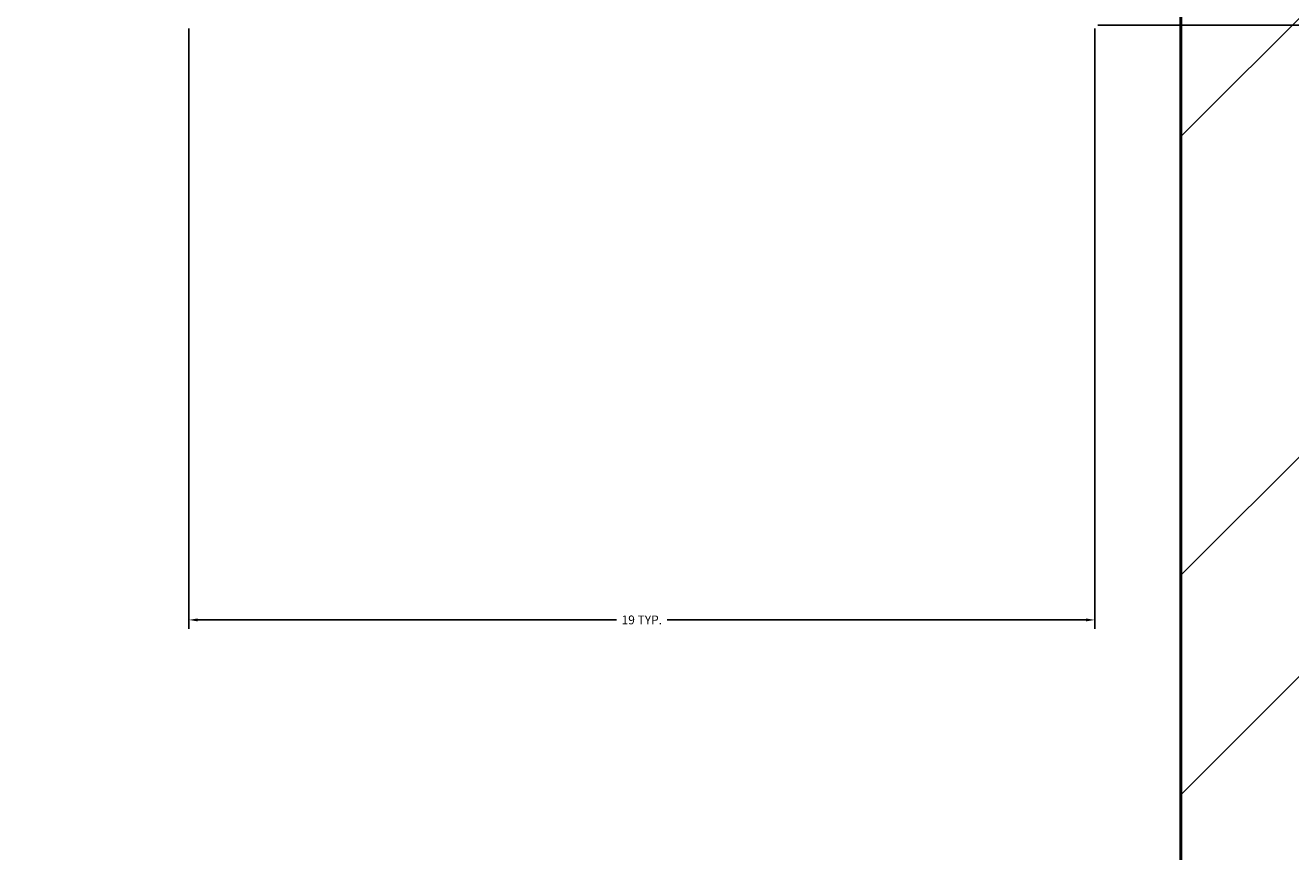
# Model space of a CAD drawing. Units: inches. Extents: x 963 to 2075, y 289 to 2657.
# Tile 20 of 98: x 1485 to 1511, y 1718 to 1735. Entities that reach past the tile are written whole.
import ezdxf

# ---------------------------------------------------------------- set-up
doc = ezdxf.new("R2010")
doc.units = ezdxf.units.IN
for name, color, linetype, lineweight in [('A-ANNO-DIMS', 2, 'Continuous', 18), ('A-WALL', 7, 'Continuous', 50), ('A-WALL-PATT', 8, 'Continuous', 13)]:
    doc.layers.add(name, color=color, linetype=linetype, lineweight=lineweight)
doc.styles.get("Standard").update_dxf_attribs({"font": 'arial.ttf'})
doc.dimstyles.get("Standard").update_dxf_attribs({"dimtxt": 0.18, "dimasz": 0.18, "dimexe": 0.18, "dimexo": 0.0625, "dimgap": 0.09, "dimtad": 0, "dimtih": 1, "dimtoh": 1, "dimdec": 4, "dimzin": 0, "dimdsep": 46, "dimtxsty": 'Standard', "dimcen": 0.09, "dimadec": 0, "dimazin": 0, "dimtfac": 1, "dimtdec": 4, "dimtofl": 0, "dimtmove": 0, "dimatfit": 3, "dimfxl": 1, "dimtolj": 1, "dimtzin": 0, "dimarcsym": 0})

# ---------------------------------------------------------------- blocks, each defined once
blk = doc.blocks.new('*D28')
at = {"layer": 'A-ANNO-DIMS', "color": 0, "lineweight": -2, "transparency": 16777216}
for p, q in [((1506.727, 1816.319), (1519.012, 1816.319)), ((1518.832, 1816.139), (1518.832, 1775.944)), ((1518.832, 1735.382), (1518.832, 1775.577)), ((1506.727, 1735.202), (1519.012, 1735.202))]:
    blk.add_line(p, q, dxfattribs=at)
at = {"layer": 'A-ANNO-DIMS', "color": 0, "transparency": 16777216}
for points in [[(1518.802, 1816.139), (1518.862, 1816.139), (1518.832, 1816.319)], [(1518.802, 1735.382), (1518.862, 1735.382), (1518.832, 1735.202)]]:
    blk.add_solid(points, dxfattribs=at)
at = {"layer": 'Defpoints', "color": 0, "transparency": 16777216}
for p in [(1506.665, 1816.319), (1518.832, 1816.319), (1506.665, 1735.202)]:
    blk.add_point(p, dxfattribs=at)
at = {"layer": 'A-ANNO-DIMS', "color": 0, "transparency": 16777216, "insert": (1518.832, 1775.761), "char_height": 0.18, "attachment_point": 5}
blk.add_mtext('\\A1;3-SEAT SOFA 81 TYP.', dxfattribs=at)
blk = doc.blocks.new('*D29')
at = {"layer": 'A-ANNO-DIMS', "color": 0, "lineweight": -2, "transparency": 16777216}
for p, q in [((1488.124, 1735.14), (1488.124, 1722.855)), ((1506.665, 1735.14), (1506.665, 1722.855)), ((1488.304, 1723.035), (1496.875, 1723.035)), ((1506.485, 1723.035), (1497.914, 1723.035))]:
    blk.add_line(p, q, dxfattribs=at)
at = {"layer": 'A-ANNO-DIMS', "color": 0, "transparency": 16777216}
for points in [[(1488.304, 1723.065), (1488.304, 1723.005), (1488.124, 1723.035)], [(1506.485, 1723.065), (1506.485, 1723.005), (1506.665, 1723.035)]]:
    blk.add_solid(points, dxfattribs=at)
at = {"layer": 'Defpoints', "color": 0, "transparency": 16777216}
for p in [(1488.124, 1735.202), (1506.665, 1735.202), (1506.665, 1723.035)]:
    blk.add_point(p, dxfattribs=at)
at = {"layer": 'A-ANNO-DIMS', "color": 0, "transparency": 16777216, "insert": (1497.394, 1723.035), "char_height": 0.18, "attachment_point": 5}
blk.add_mtext('\\A1;19 TYP.', dxfattribs=at)

msp = doc.modelspace()

# ---------------------------------------------------------------- hatches: boundary and pattern name
at = {"layer": 'A-WALL-PATT'}
h = msp.add_hatch(dxfattribs=at)
h.set_pattern_fill('ANSI32', color=256)
h.paths.add_polyline_path([(1473.609, 2163.068), (1473.609, 2165.318), (1376.422, 2165.318), (1376.422, 2227.983), (1371.922, 2227.983), (1371.922, 2214.818), (1368.405, 2214.818), (1368.405, 2210.318), (1371.922, 2210.318), (1371.922, 2160.818), (1395.922, 2160.818), (1395.922, 2090.318), (1217.345, 2090.318), (1217.345, 2085.818), (1395.922, 2085.818), (1458.922, 2085.818), (1458.922, 2108.318), (1454.422, 2108.318), (1454.422, 2090.318), (1400.422, 2090.318), (1400.422, 2160.818), (1473.609, 2160.818)])
h.paths.add_polyline_path([(1649.422, 2210.318), (1653.225, 2210.318), (1653.225, 2214.818), (1649.422, 2214.818), (1649.422, 2227.983), (1644.922, 2227.983), (1644.922, 2165.318), (1550.099, 2165.318), (1550.099, 2160.818), (1620.922, 2160.818), (1620.922, 2112.818), (1555.446, 2112.818), (1555.446, 2108.318), (1584.327, 2108.318), (1584.327, 2084.916), (1588.827, 2084.916), (1588.827, 2108.318), (1625.422, 2108.318), (1667.951, 2108.318), (1667.951, 2022.667), (1588.827, 2022.667), (1588.827, 2047.408), (1584.327, 2047.408), (1584.327, 1996.003), (1588.827, 1996.003), (1588.827, 2018.318), (1667.951, 2018.167), (1667.951, 1928.318), (1625.422, 1928.318), (1625.422, 1923.818), (1672.451, 1923.818), (1672.451, 1928.318), (1672.451, 1946.663), (1785.446, 1946.663), (1785.446, 1951.163), (1743.034, 1951.163), (1743.034, 2017.922), (1841.422, 2017.922), (1841.422, 2014.775), (1845.922, 2014.775), (1845.922, 2017.922), (1905.922, 2017.922), (1905.922, 1987.511), (1910.422, 1987.511), (1910.422, 2022.422), (1910.422, 2068.517), (1905.922, 2068.517), (1905.922, 2022.422), (1845.922, 2022.422), (1845.922, 2025.851), (1843.672, 2025.851), (1841.422, 2025.851), (1841.422, 2022.422), (1743.034, 2022.422), (1743.034, 2084.031), (1768.451, 2084.031), (1785.446, 2084.031), (1785.446, 2088.531), (1672.451, 2088.531), (1672.451, 2112.818), (1667.951, 2112.818), (1625.422, 2112.818), (1625.422, 2160.818), (1649.422, 2160.818)])
h.paths.add_polyline_path([(1672.451, 2084.031), (1738.534, 2084.031), (1738.534, 1951.163), (1672.451, 1951.163)], flags=16)
h.paths.add_polyline_path([(1672.451, 2084.031), (1738.534, 2084.031), (1705.492, 2017.597)], flags=0)
h.paths.add_polyline_path([(1262.766, 2085.818), (1258.266, 2085.818), (1258.266, 2023.278), (1184.422, 2023.278), (1184.422, 2018.778), (1258.266, 2018.778), (1258.266, 1950.818), (1262.766, 1950.818)])
h.paths.add_polyline_path([(1312.266, 2085.818), (1307.766, 2085.818), (1307.766, 1950.818), (1312.266, 1950.818)])
h.paths.add_polyline_path([(1458.922, 1950.818), (1395.922, 1950.818), (1216.568, 1950.818), (1216.568, 1946.318), (1346.422, 1946.318), (1395.922, 1946.318), (1395.922, 1875.818), (1371.922, 1875.818), (1371.922, 1826.318), (1368.931, 1826.318), (1368.931, 1821.818), (1371.922, 1821.818), (1371.922, 1813.622), (1376.422, 1813.622), (1376.422, 1871.318), (1474.504, 1871.318), (1474.504, 1873.568), (1474.504, 1875.818), (1400.422, 1875.818), (1400.422, 1946.318), (1454.422, 1946.318), (1454.422, 1928.318), (1458.922, 1928.318)])
h.paths.add_polyline_path([(1184.422, 2120.778), (1167.922, 2120.778), (1167.922, 2134.812), (1165.672, 2134.812), (1163.422, 2134.812), (1163.422, 2120.778), (1119.922, 2120.778), (1119.922, 2098.095), (1124.422, 2098.095), (1124.422, 2116.278), (1167.922, 2116.278), (1179.922, 2116.278), (1179.922, 2045.916), (1184.422, 2045.916), (1184.422, 2090.318), (1184.422, 2116.278)])
h.paths.add_polyline_path([(1124.422, 2018.778), (1179.922, 2018.778), (1179.922, 2016.294), (1184.422, 2016.294), (1184.422, 2023.278), (1184.422, 2026.588), (1182.172, 2026.588), (1179.922, 2026.588), (1179.922, 2023.278), (1124.422, 2023.278), (1124.422, 2074.095), (1119.922, 2074.095), (1119.922, 2018.778), (1119.922, 1979.633), (1124.422, 1979.633)])
h.paths.add_polyline_path([(1184.422, 1925.778), (1184.422, 1946.318), (1184.422, 1996.073), (1182.172, 1996.073), (1179.922, 1996.073), (1179.922, 1925.778), (1124.422, 1925.778), (1124.422, 1955.633), (1119.922, 1955.502), (1119.922, 1921.278), (1158.922, 1921.278), (1158.922, 1909.983), (1163.422, 1909.983), (1163.422, 1921.278), (1184.422, 1921.278)])
h.paths.add_polyline_path([(1341.449, 1826.318), (1163.422, 1826.318), (1163.422, 1849.983), (1158.922, 1849.983), (1158.922, 1821.818), (1158.922, 1804.033), (1163.422, 1804.033), (1163.422, 1821.818), (1341.449, 1821.818)])
h.paths.add_polyline_path([(1222.981, 1713.818), (1163.422, 1713.818), (1163.422, 1744.033), (1161.172, 1744.033), (1158.922, 1744.033), (1158.922, 1713.818), (1119.922, 1713.818), (1119.922, 1694.65), (1124.422, 1694.65), (1124.422, 1709.318), (1158.922, 1709.318), (1222.981, 1709.318)])
h.paths.add_polyline_path([(1328.422, 1713.818), (1252.042, 1713.818), (1252.042, 1711.568), (1252.042, 1709.318), (1256.422, 1709.318), (1256.422, 1547.318), (1232.937, 1547.318), (1232.937, 1545.068), (1232.937, 1542.818), (1292.422, 1542.818), (1292.422, 1527.634), (1296.922, 1527.634), (1296.922, 1542.818), (1299.464, 1542.818), (1299.464, 1547.318), (1260.922, 1547.318), (1260.922, 1658.318), (1343.661, 1658.318), (1343.661, 1660.568), (1343.661, 1662.818), (1328.422, 1662.818), (1328.422, 1676.589), (1327.402, 1676.589), (1323.922, 1676.589), (1323.922, 1662.818), (1260.922, 1662.818), (1260.922, 1709.318), (1323.922, 1709.318), (1323.922, 1699.851), (1328.422, 1699.851)])
h.paths.add_polyline_path([(1649.422, 1875.818), (1625.422, 1875.818), (1625.422, 1928.318), (1620.922, 1928.318), (1588.827, 1928.318), (1588.827, 1950.59), (1584.327, 1950.59), (1584.327, 1928.318), (1555.446, 1928.318), (1555.446, 1923.818), (1620.922, 1923.818), (1620.922, 1875.818), (1548.952, 1875.818), (1548.952, 1873.568), (1548.952, 1871.318), (1644.922, 1871.318), (1644.922, 1813.622), (1649.422, 1813.622), (1649.422, 1821.818), (1652.045, 1821.818), (1652.045, 1824.068), (1652.045, 1826.318), (1649.422, 1826.318)])
h.paths.add_polyline_path([(1512.922, 1871.318), (1516.476, 1871.318), (1516.476, 1875.818), (1512.922, 1875.818), (1512.922, 1923.818), (1512.922, 1928.318), (1512.922, 1930.827), (1508.422, 1930.827), (1508.422, 1875.818), (1504.411, 1875.818), (1504.411, 1871.318), (1508.422, 1871.318), (1508.422, 1713.818), (1376.422, 1713.818), (1376.422, 1743.325), (1371.922, 1743.325), (1371.922, 1709.318), (1371.922, 1706.01), (1376.422, 1706.01), (1376.422, 1709.318), (1508.422, 1709.318), (1508.422, 1547.318), (1501.871, 1547.318), (1501.871, 1542.818), (1508.422, 1542.818), (1508.422, 1482.818), (1508.422, 1436.318), (1512.922, 1436.318), (1512.922, 1542.818), (1519.318, 1542.818), (1519.318, 1545.068), (1519.318, 1547.318), (1512.922, 1547.318), (1512.922, 1709.318), (1644.922, 1709.318), (1644.922, 1707.548), (1649.422, 1707.548), (1649.422, 1709.318), (1649.422, 1743.325), (1644.922, 1743.325), (1644.922, 1713.818), (1512.922, 1713.818)])
h.paths.add_polyline_path([(1129.884, 1545.068), (1129.884, 1547.318), (1124.422, 1547.318), (1095.922, 1547.318), (1095.922, 1614.818), (1124.422, 1614.818), (1124.422, 1619.318), (1095.922, 1619.318), (1091.422, 1619.318), (1091.422, 1542.818), (1095.922, 1542.818), (1119.922, 1542.818), (1129.884, 1542.818)])
h.paths.add_polyline_path([(1208.422, 1542.818), (1211.74, 1542.818), (1211.74, 1547.318), (1198.851, 1547.318), (1198.851, 1542.818), (1203.922, 1542.818), (1203.922, 1478.318), (1208.422, 1478.318), (1296.922, 1478.318), (1296.922, 1503.634), (1292.422, 1503.634), (1292.422, 1482.818), (1208.422, 1482.818)])
h.paths.add_polyline_path([(1430.422, 1542.818), (1435.699, 1542.818), (1435.699, 1545.068), (1435.699, 1547.318), (1422.658, 1547.318), (1422.658, 1545.068), (1422.658, 1542.818), (1425.922, 1542.818), (1425.922, 1482.857), (1341.922, 1482.857), (1341.922, 1502.732), (1337.422, 1502.732), (1337.422, 1478.357), (1425.922, 1478.357), (1425.922, 1440.818), (1425.922, 1436.318), (1430.422, 1436.318)])
h.paths.add_polyline_path([(1698.482, 2004.259), (1727.695, 2004.259), (1727.695, 2022.916), (1698.482, 2022.916)], flags=8)

# ---------------------------------------------------------------- linework, layer by layer
at = {"layer": 'A-WALL'}
msp.add_line((1508.422, 1871.318), (1508.422, 1713.818), dxfattribs=at)

# ---------------------------------------------------------------- dimensions: what is measured, and where the dimension line sits
at = {"layer": 'A-ANNO-DIMS'}
dim = msp.add_linear_dim(base=(1518.832, 1816.319), p1=(1506.665, 1735.202), p2=(1506.665, 1816.319), angle=90, text='3-SEAT SOFA <> TYP.', dimstyle='Standard', override={"dimdec": 0, "dimlfac": 1, "dimrnd": 0, "dimzin": 0, "dimdsep": 46, "dimlunit": 2}, dxfattribs=at)
dim.commit()
dim.dimension.update_dxf_attribs({"geometry": '*D28', "text_midpoint": (1518.832, 1775.761)})
dim = msp.add_linear_dim(base=(1506.665, 1723.035), p1=(1488.124, 1735.202), p2=(1506.665, 1735.202), text='<> TYP.', dimstyle='Standard', override={"dimdec": 0, "dimlfac": 1, "dimrnd": 0, "dimzin": 0, "dimdsep": 46, "dimlunit": 2}, dxfattribs=at)
dim.commit()
dim.dimension.update_dxf_attribs({"geometry": '*D29', "text_midpoint": (1497.394, 1723.035)})

doc.saveas('drawing.dxf')
